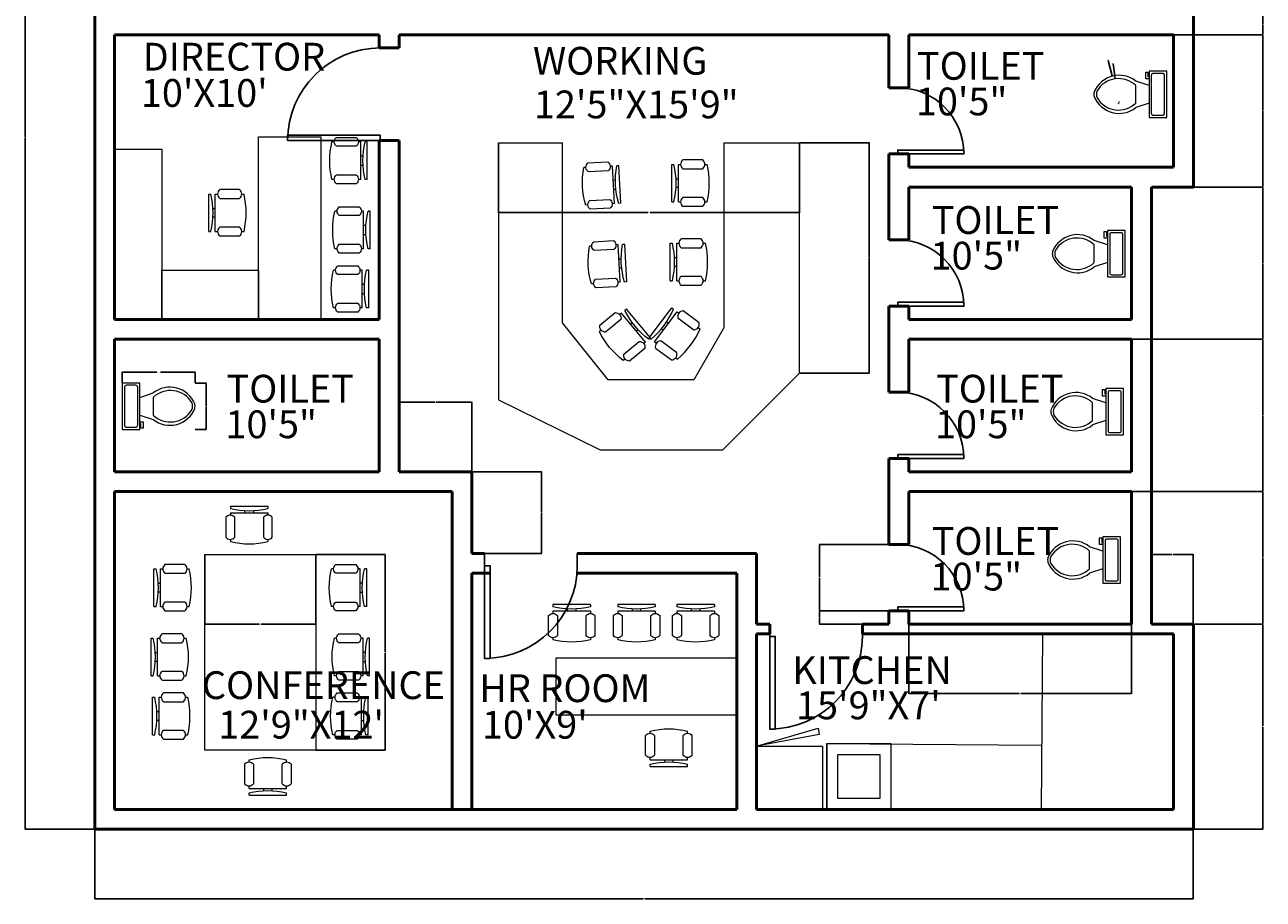
# Model space of a CAD drawing. Units: inches. Extents: x 4242 to 4803, y 4687 to 5377.
# Tile 1 of 2: x 4242 to 4803, y 4687 to 5083. Entities that reach past the tile are written whole.
import ezdxf

# ---------------------------------------------------------------- set-up
doc = ezdxf.new("R2010")
doc.units = ezdxf.units.IN
for name, color, linetype, lineweight in [('A-ANNO-DIMS', 2, 'Continuous', 18), ('A-AREA-IDEN', 7, 'Continuous', 25), ('A-DOOR', 4, 'Continuous', 25), ('A-FLOR-FIXT', 9, 'Continuous', 18), ('A-FURN', 8, 'Continuous', 18), ('A-WALL', 7, 'Continuous', 50)]:
    doc.layers.add(name, color=color, linetype=linetype, lineweight=lineweight)
doc.styles.get("Standard").update_dxf_attribs({"font": 'arial.ttf'})
doc.dimstyles.get("Standard").update_dxf_attribs({"dimtxt": 0.18, "dimasz": 0.18, "dimexe": 0.18, "dimexo": 0.0625, "dimgap": 0.09, "dimtad": 0, "dimtih": 1, "dimtoh": 1, "dimdec": 4, "dimzin": 0, "dimdsep": 46, "dimtxsty": 'Standard', "dimcen": 0.09, "dimadec": 0, "dimazin": 0, "dimtfac": 1, "dimtdec": 4, "dimtofl": 0, "dimtmove": 0, "dimatfit": 3, "dimfxl": 1, "dimtolj": 1, "dimtzin": 0, "dimarcsym": 0})

# ---------------------------------------------------------------- blocks, each defined once
blk = doc.blocks.new('Toilet - top')
for p, q in [((9.5, -6), (9.5, -2)), ((-10, -8.5), (-8, -8.5)), ((-10, -9.5), (-10, -8.5)), ((-7, -9.5), (-10, -9.5)), ((-8, -8.5), (-8, -8)), ((-7, -8), (-7, -9.5)), ((-4, -8), (-6, -14)), ((4, -8), (6, -14)), ((4, -14), (-4, -14))]:
    blk.add_line(p, q)
blk.add_lwpolyline([(10.5, -8), (10.5, 0), (-10.5, 0), (-10.5, -8)], close=True)
for points in [[(-9.5, -2), (-9.5, -6)], [(8.5, -1), (-8.5, -1)], [(-8.5, -7), (8.5, -7)]]:
    blk.add_lwpolyline(points)
for centre, radius, start, end in [((-8.62, -1.88), 0.884, 81.8699, 188.1301), ((8.62, -1.88), 0.884, 351.8699, 98.1301), ((-8.62, -6.12), 0.884, 171.8699, 278.1301), ((8.62, -6.12), 0.884, 261.8699, 8.1301), ((3.52, -21.58), 12.17, 141.4691, 247.9714), ((4.2, -21.82), 11.33, 136.3677, 238.9468), ((-3.52, -21.58), 12.17, 292.0284, 38.5307), ((-4.2, -21.82), 11.33, 301.053, 43.6321), ((0, -27.88), 4, 245.7318, 294.2682), ((0, -29), 4, 254.8605, 285.1395)]:
    blk.add_arc(centre, radius, start, end)
blk = doc.blocks.new('Chair - Desk')
for p, q in [((-8.5, 0), (-8.5, -1)), ((-8.5, 0), (8.5, 0)), ((8.5, 0), (8.5, -1)), ((-10.5, -5), (-10.5, -14)), ((-8.5, -3), (-8.5, -4)), ((-8.5, -3), (8.5, -3)), ((-6.5, -14), (-6.5, -5)), ((-2, -3), (-2, -1.9355)), ((2, -1.9576), (2, -3)), ((6.5, -5), (6.5, -14)), ((8.5, -3), (8.5, -4)), ((10.5, -14), (10.5, -5)), ((-8.5, -15), (-8.5, -16)), ((8.5, -15), (8.5, -16))]:
    blk.add_line(p, q)
for centre, radius, start, end in [((-8.5, -6.5), 2.5, 36.8699, 143.1301), ((0, 34.625), 36.625, 256.5803, 283.4197), ((8.5, -6.5), 2.5, 36.8699, 143.1301), ((-8.5, -12.5), 2.5, 216.8699, 323.1301), ((0, 19.625), 36.625, 256.5803, 283.4197), ((8.5, -12.5), 2.5, 216.8699, 323.1301)]:
    blk.add_arc(centre, radius, start, end)
blk = doc.blocks.new('*U4')
for p, q in [((0, 0), (0, -100)), ((750, 0), (750, -100))]:
    blk.add_line(p, q)
blk.add_lwpolyline([(0, 0), (0, 750), (43.75, 750), (43.75, 0)], close=True)
blk.add_arc((0, 0), 750, 0, 90)
blk = doc.blocks.new('*D8')
at = {"layer": 'A-ANNO-DIMS', "color": 0, "lineweight": -2, "transparency": 16777216}
for p, q in [((4285.76, 4920.88), (4285.76, 4925.95)), ((4285.94, 4925.77), (4301.51, 4925.77)), ((4318.63, 4925.77), (4303.06, 4925.77)), ((4318.81, 4920.88), (4318.81, 4925.95))]:
    blk.add_line(p, q, dxfattribs=at)
at = {"layer": 'A-ANNO-DIMS', "color": 0, "transparency": 16777216}
for points in [[(4285.94, 4925.8), (4285.94, 4925.74), (4285.76, 4925.77)], [(4318.63, 4925.8), (4318.63, 4925.74), (4318.81, 4925.77)]]:
    blk.add_solid(points, dxfattribs=at)
at = {"layer": 'Defpoints', "color": 0, "transparency": 16777216}
for p in [(4285.76, 4925.77), (4285.76, 4920.82), (4318.81, 4920.82)]:
    blk.add_point(p, dxfattribs=at)
at = {"layer": 'A-ANNO-DIMS', "color": 0, "transparency": 16777216, "insert": (4302.29, 4925.77), "char_height": 0.18, "attachment_point": 5}
blk.add_mtext('\\A1;WC 33 TYP.', dxfattribs=at)
blk = doc.blocks.new('*D9')
at = {"layer": 'A-ANNO-DIMS', "color": 0, "lineweight": -2, "transparency": 16777216}
for p, q in [((4318.87, 4920.82), (4323.95, 4920.82)), ((4323.77, 4920.64), (4323.77, 4910.5)), ((4323.77, 4900), (4323.77, 4910.14)), ((4318.87, 4899.82), (4323.95, 4899.82))]:
    blk.add_line(p, q, dxfattribs=at)
at = {"layer": 'A-ANNO-DIMS', "color": 0, "transparency": 16777216}
for points in [[(4323.74, 4920.64), (4323.8, 4920.64), (4323.77, 4920.82)], [(4323.74, 4900), (4323.8, 4900), (4323.77, 4899.82)]]:
    blk.add_solid(points, dxfattribs=at)
at = {"layer": 'Defpoints', "color": 0, "transparency": 16777216}
for p in [(4318.81, 4920.82), (4323.77, 4920.82), (4318.81, 4899.82)]:
    blk.add_point(p, dxfattribs=at)
at = {"layer": 'A-ANNO-DIMS', "color": 0, "transparency": 16777216, "insert": (4323.77, 4910.32), "char_height": 0.18, "attachment_point": 5}
blk.add_mtext('\\A1;21 TYP.', dxfattribs=at)
blk = doc.blocks.new('*D12')
at = {"layer": 'A-ANNO-DIMS', "color": 0, "lineweight": -2, "transparency": 16777216}
for p, q in [((4273.28, 4718.58), (4273.28, 4686.96)), ((4771.28, 4718.58), (4771.28, 4686.96)), ((4273.46, 4687.14), (4521.99, 4687.14)), ((4771.1, 4687.14), (4522.58, 4687.14))]:
    blk.add_line(p, q, dxfattribs=at)
at = {"layer": 'A-ANNO-DIMS', "color": 0, "transparency": 16777216}
for points in [[(4273.46, 4687.17), (4273.46, 4687.11), (4273.28, 4687.14)], [(4771.1, 4687.17), (4771.1, 4687.11), (4771.28, 4687.14)]]:
    blk.add_solid(points, dxfattribs=at)
at = {"layer": 'Defpoints', "color": 0, "transparency": 16777216}
for p in [(4273.28, 4718.64), (4771.28, 4718.64), (4771.28, 4687.14)]:
    blk.add_point(p, dxfattribs=at)
at = {"layer": 'A-ANNO-DIMS', "color": 0, "transparency": 16777216, "insert": (4522.28, 4687.14), "char_height": 0.18, "attachment_point": 5}
blk.add_mtext('\\A1;498', dxfattribs=at)
blk = doc.blocks.new('*D13')
at = {"layer": 'A-ANNO-DIMS', "color": 0, "lineweight": -2, "transparency": 16777216}
for p, q in [((4633.22, 5345.64), (4241.6, 5345.64)), ((4241.78, 5345.46), (4241.78, 5032.32)), ((4241.78, 4718.82), (4241.78, 5031.96)), ((4273.22, 4718.64), (4241.6, 4718.64))]:
    blk.add_line(p, q, dxfattribs=at)
at = {"layer": 'A-ANNO-DIMS', "color": 0, "transparency": 16777216}
for points in [[(4241.75, 5345.46), (4241.81, 5345.46), (4241.78, 5345.64)], [(4241.75, 4718.82), (4241.81, 4718.82), (4241.78, 4718.64)]]:
    blk.add_solid(points, dxfattribs=at)
at = {"layer": 'Defpoints', "color": 0, "transparency": 16777216}
for p in [(4241.78, 5345.64), (4633.28, 5345.64), (4273.28, 4718.64)]:
    blk.add_point(p, dxfattribs=at)
at = {"layer": 'A-ANNO-DIMS', "color": 0, "transparency": 16777216, "insert": (4241.78, 5032.14), "char_height": 0.18, "attachment_point": 5}
blk.add_mtext('\\A1;627', dxfattribs=at)
blk = doc.blocks.new('*D16')
at = {"layer": 'A-ANNO-DIMS', "color": 0, "lineweight": -2, "transparency": 16777216}
for p, q in [((4771.35, 4811.64), (4802.96, 4811.64)), ((4802.78, 4811.46), (4802.78, 4765.32)), ((4802.78, 4718.82), (4802.78, 4764.96)), ((4771.35, 4718.64), (4802.96, 4718.64))]:
    blk.add_line(p, q, dxfattribs=at)
at = {"layer": 'A-ANNO-DIMS', "color": 0, "transparency": 16777216}
for points in [[(4802.75, 4811.46), (4802.81, 4811.46), (4802.78, 4811.64)], [(4802.75, 4718.82), (4802.81, 4718.82), (4802.78, 4718.64)]]:
    blk.add_solid(points, dxfattribs=at)
at = {"layer": 'Defpoints', "color": 0, "transparency": 16777216}
for p in [(4771.28, 4811.64), (4802.78, 4811.64), (4771.28, 4718.64)]:
    blk.add_point(p, dxfattribs=at)
at = {"layer": 'A-ANNO-DIMS', "color": 0, "transparency": 16777216, "insert": (4802.78, 4765.14), "char_height": 0.18, "attachment_point": 5}
blk.add_mtext('\\A1;93', dxfattribs=at)
blk = doc.blocks.new('*D17')
at = {"layer": 'A-ANNO-DIMS', "color": 0, "lineweight": -2, "transparency": 16777216}
for p, q in [((4743.35, 4871.64), (4802.96, 4871.64)), ((4802.78, 4871.46), (4802.78, 4841.82)), ((4802.78, 4811.82), (4802.78, 4841.46)), ((4752.35, 4811.64), (4802.96, 4811.64))]:
    blk.add_line(p, q, dxfattribs=at)
at = {"layer": 'A-ANNO-DIMS', "color": 0, "transparency": 16777216}
for points in [[(4802.75, 4871.46), (4802.81, 4871.46), (4802.78, 4871.64)], [(4802.75, 4811.82), (4802.81, 4811.82), (4802.78, 4811.64)]]:
    blk.add_solid(points, dxfattribs=at)
at = {"layer": 'Defpoints', "color": 0, "transparency": 16777216}
for p in [(4743.28, 4871.64), (4802.78, 4871.64), (4752.28, 4811.64)]:
    blk.add_point(p, dxfattribs=at)
at = {"layer": 'A-ANNO-DIMS', "color": 0, "transparency": 16777216, "insert": (4802.78, 4841.64), "char_height": 0.18, "attachment_point": 5}
blk.add_mtext('\\A1;60', dxfattribs=at)
blk = doc.blocks.new('*D18')
at = {"layer": 'A-ANNO-DIMS', "color": 0, "lineweight": -2, "transparency": 16777216}
for p, q in [((4743.35, 4940.64), (4802.96, 4940.64)), ((4802.78, 4940.46), (4802.78, 4906.32)), ((4802.78, 4871.82), (4802.78, 4905.96)), ((4743.35, 4871.64), (4802.96, 4871.64))]:
    blk.add_line(p, q, dxfattribs=at)
at = {"layer": 'A-ANNO-DIMS', "color": 0, "transparency": 16777216}
for points in [[(4802.75, 4940.46), (4802.81, 4940.46), (4802.78, 4940.64)], [(4802.75, 4871.82), (4802.81, 4871.82), (4802.78, 4871.64)]]:
    blk.add_solid(points, dxfattribs=at)
at = {"layer": 'Defpoints', "color": 0, "transparency": 16777216}
for p in [(4743.28, 4940.64), (4802.78, 4940.64), (4743.28, 4871.64)]:
    blk.add_point(p, dxfattribs=at)
at = {"layer": 'A-ANNO-DIMS', "color": 0, "transparency": 16777216, "insert": (4802.78, 4906.14), "char_height": 0.18, "attachment_point": 5}
blk.add_mtext('\\A1;69', dxfattribs=at)
blk = doc.blocks.new('*D19')
at = {"layer": 'A-ANNO-DIMS', "color": 0, "lineweight": -2, "transparency": 16777216}
for p, q in [((4752.35, 5009.64), (4802.96, 5009.64)), ((4802.78, 5009.46), (4802.78, 4975.32)), ((4802.78, 4940.82), (4802.78, 4974.96)), ((4743.35, 4940.64), (4802.96, 4940.64))]:
    blk.add_line(p, q, dxfattribs=at)
at = {"layer": 'A-ANNO-DIMS', "color": 0, "transparency": 16777216}
for points in [[(4802.75, 5009.46), (4802.81, 5009.46), (4802.78, 5009.64)], [(4802.75, 4940.82), (4802.81, 4940.82), (4802.78, 4940.64)]]:
    blk.add_solid(points, dxfattribs=at)
at = {"layer": 'Defpoints', "color": 0, "transparency": 16777216}
for p in [(4752.28, 5009.64), (4802.78, 5009.64), (4743.28, 4940.64)]:
    blk.add_point(p, dxfattribs=at)
at = {"layer": 'A-ANNO-DIMS', "color": 0, "transparency": 16777216, "insert": (4802.78, 4975.14), "char_height": 0.18, "attachment_point": 5}
blk.add_mtext('\\A1;69', dxfattribs=at)
blk = doc.blocks.new('*D20')
at = {"layer": 'A-ANNO-DIMS', "color": 0, "lineweight": -2, "transparency": 16777216}
for p, q in [((4762.35, 5078.64), (4802.96, 5078.64)), ((4802.78, 5078.46), (4802.78, 5044.32)), ((4802.78, 5009.82), (4802.78, 5043.96)), ((4771.35, 5009.64), (4802.96, 5009.64))]:
    blk.add_line(p, q, dxfattribs=at)
at = {"layer": 'A-ANNO-DIMS', "color": 0, "transparency": 16777216}
for points in [[(4802.75, 5078.46), (4802.81, 5078.46), (4802.78, 5078.64)], [(4802.75, 5009.82), (4802.81, 5009.82), (4802.78, 5009.64)]]:
    blk.add_solid(points, dxfattribs=at)
at = {"layer": 'Defpoints', "color": 0, "transparency": 16777216}
for p in [(4762.28, 5078.64), (4802.78, 5078.64), (4771.28, 5009.64)]:
    blk.add_point(p, dxfattribs=at)
at = {"layer": 'A-ANNO-DIMS', "color": 0, "transparency": 16777216, "insert": (4802.78, 5044.14), "char_height": 0.18, "attachment_point": 5}
blk.add_mtext('\\A1;69', dxfattribs=at)
blk = doc.blocks.new('*D21')
at = {"layer": 'A-ANNO-DIMS', "color": 0, "lineweight": -2, "transparency": 16777216}
for p, q in [((4762.35, 5087.64), (4802.96, 5087.64)), ((4802.78, 5087.46), (4802.78, 5083.32)), ((4802.78, 5078.82), (4802.78, 5082.96)), ((4762.35, 5078.64), (4802.96, 5078.64))]:
    blk.add_line(p, q, dxfattribs=at)
at = {"layer": 'A-ANNO-DIMS', "color": 0, "transparency": 16777216}
for points in [[(4802.75, 5087.46), (4802.81, 5087.46), (4802.78, 5087.64)], [(4802.75, 5078.82), (4802.81, 5078.82), (4802.78, 5078.64)]]:
    blk.add_solid(points, dxfattribs=at)
at = {"layer": 'Defpoints', "color": 0, "transparency": 16777216}
for p in [(4762.28, 5087.64), (4802.78, 5087.64), (4762.28, 5078.64)]:
    blk.add_point(p, dxfattribs=at)
at = {"layer": 'A-ANNO-DIMS', "color": 0, "transparency": 16777216, "insert": (4802.78, 5083.14), "char_height": 0.18, "attachment_point": 5}
blk.add_mtext('\\A1;9', dxfattribs=at)
blk = doc.blocks.new('*D25')
at = {"layer": 'A-ANNO-DIMS', "color": 0, "lineweight": -2, "transparency": 16777216}
for p, q in [((4752.28, 4811.7), (4752.28, 4843.32)), ((4752.46, 4843.14), (4761.57, 4843.14)), ((4771.1, 4843.14), (4762, 4843.14)), ((4771.28, 4811.7), (4771.28, 4843.32))]:
    blk.add_line(p, q, dxfattribs=at)
at = {"layer": 'A-ANNO-DIMS', "color": 0, "transparency": 16777216}
for points in [[(4752.46, 4843.17), (4752.46, 4843.11), (4752.28, 4843.14)], [(4771.1, 4843.17), (4771.1, 4843.11), (4771.28, 4843.14)]]:
    blk.add_solid(points, dxfattribs=at)
at = {"layer": 'Defpoints', "color": 0, "transparency": 16777216}
for p in [(4771.28, 4843.14), (4752.28, 4811.64), (4771.28, 4811.64)]:
    blk.add_point(p, dxfattribs=at)
at = {"layer": 'A-ANNO-DIMS', "color": 0, "transparency": 16777216, "insert": (4761.78, 4843.14), "char_height": 0.18, "attachment_point": 5}
blk.add_mtext('\\A1;19', dxfattribs=at)
blk = doc.blocks.new('*D28')
at = {"layer": 'A-ANNO-DIMS', "color": 0, "lineweight": -2, "transparency": 16777216}
for p, q in [((4633.22, 4847.64), (4601.6, 4847.64)), ((4601.78, 4847.46), (4601.78, 4832.82)), ((4601.78, 4817.82), (4601.78, 4832.46)), ((4633.22, 4817.64), (4601.6, 4817.64))]:
    blk.add_line(p, q, dxfattribs=at)
at = {"layer": 'A-ANNO-DIMS', "color": 0, "transparency": 16777216}
for points in [[(4601.75, 4847.46), (4601.81, 4847.46), (4601.78, 4847.64)], [(4601.75, 4817.82), (4601.81, 4817.82), (4601.78, 4817.64)]]:
    blk.add_solid(points, dxfattribs=at)
at = {"layer": 'Defpoints', "color": 0, "transparency": 16777216}
for p in [(4601.78, 4847.64), (4633.28, 4847.64), (4633.28, 4817.64)]:
    blk.add_point(p, dxfattribs=at)
at = {"layer": 'A-ANNO-DIMS', "color": 0, "transparency": 16777216, "insert": (4601.78, 4832.64), "char_height": 0.18, "attachment_point": 5}
blk.add_mtext('\\A1;30', dxfattribs=at)
blk = doc.blocks.new('*D29')
at = {"layer": 'A-ANNO-DIMS', "color": 0, "lineweight": -2, "transparency": 16777216}
for p, q in [((4633.22, 4817.64), (4601.6, 4817.64)), ((4601.78, 4817.46), (4601.78, 4814.82)), ((4633.22, 4811.64), (4601.6, 4811.64)), ((4601.78, 4811.82), (4601.78, 4814.46))]:
    blk.add_line(p, q, dxfattribs=at)
at = {"layer": 'A-ANNO-DIMS', "color": 0, "transparency": 16777216}
for points in [[(4601.75, 4817.46), (4601.81, 4817.46), (4601.78, 4817.64)], [(4601.75, 4811.82), (4601.81, 4811.82), (4601.78, 4811.64)]]:
    blk.add_solid(points, dxfattribs=at)
at = {"layer": 'Defpoints', "color": 0, "transparency": 16777216}
for p in [(4601.78, 4817.64), (4633.28, 4817.64), (4633.28, 4811.64)]:
    blk.add_point(p, dxfattribs=at)
at = {"layer": 'A-ANNO-DIMS', "color": 0, "transparency": 16777216, "insert": (4601.78, 4814.64), "char_height": 0.18, "attachment_point": 5}
blk.add_mtext('\\A1;6', dxfattribs=at)
blk = doc.blocks.new('*D32')
at = {"layer": 'A-ANNO-DIMS', "color": 0, "lineweight": -2, "transparency": 16777216}
for p, q in [((4642.28, 4811.58), (4642.28, 4779.96)), ((4743.28, 4811.58), (4743.28, 4779.96)), ((4642.46, 4780.14), (4692.52, 4780.14)), ((4743.1, 4780.14), (4693.05, 4780.14))]:
    blk.add_line(p, q, dxfattribs=at)
at = {"layer": 'A-ANNO-DIMS', "color": 0, "transparency": 16777216}
for points in [[(4642.46, 4780.17), (4642.46, 4780.11), (4642.28, 4780.14)], [(4743.1, 4780.17), (4743.1, 4780.11), (4743.28, 4780.14)]]:
    blk.add_solid(points, dxfattribs=at)
at = {"layer": 'Defpoints', "color": 0, "transparency": 16777216}
for p in [(4642.28, 4811.64), (4743.28, 4811.64), (4642.28, 4780.14)]:
    blk.add_point(p, dxfattribs=at)
at = {"layer": 'A-ANNO-DIMS', "color": 0, "transparency": 16777216, "insert": (4692.78, 4780.14), "char_height": 0.18, "attachment_point": 5}
blk.add_mtext('\\A1;101', dxfattribs=at)
blk = doc.blocks.new('*D33')
at = {"layer": 'A-ANNO-DIMS', "color": 0, "lineweight": -2, "transparency": 16777216}
for p, q in [((4411.28, 4880.7), (4411.28, 4912.32)), ((4411.46, 4912.14), (4427.57, 4912.14)), ((4444.1, 4912.14), (4428, 4912.14)), ((4444.28, 4880.7), (4444.28, 4912.32))]:
    blk.add_line(p, q, dxfattribs=at)
at = {"layer": 'A-ANNO-DIMS', "color": 0, "transparency": 16777216}
for points in [[(4411.46, 4912.17), (4411.46, 4912.11), (4411.28, 4912.14)], [(4444.1, 4912.17), (4444.1, 4912.11), (4444.28, 4912.14)]]:
    blk.add_solid(points, dxfattribs=at)
at = {"layer": 'Defpoints', "color": 0, "transparency": 16777216}
for p in [(4444.28, 4912.14), (4411.28, 4880.64), (4444.28, 4880.64)]:
    blk.add_point(p, dxfattribs=at)
at = {"layer": 'A-ANNO-DIMS', "color": 0, "transparency": 16777216, "insert": (4427.78, 4912.14), "char_height": 0.18, "attachment_point": 5}
blk.add_mtext('\\A1;33', dxfattribs=at)
blk = doc.blocks.new('*D34')
at = {"layer": 'A-ANNO-DIMS', "color": 0, "lineweight": -2, "transparency": 16777216}
for p, q in [((4444.35, 4880.64), (4475.96, 4880.64)), ((4475.78, 4880.46), (4475.78, 4862.32)), ((4475.78, 4843.82), (4475.78, 4861.96)), ((4444.35, 4843.64), (4475.96, 4843.64))]:
    blk.add_line(p, q, dxfattribs=at)
at = {"layer": 'A-ANNO-DIMS', "color": 0, "transparency": 16777216}
for points in [[(4475.75, 4880.46), (4475.81, 4880.46), (4475.78, 4880.64)], [(4475.75, 4843.82), (4475.81, 4843.82), (4475.78, 4843.64)]]:
    blk.add_solid(points, dxfattribs=at)
at = {"layer": 'Defpoints', "color": 0, "transparency": 16777216}
for p in [(4444.28, 4880.64), (4444.28, 4843.64), (4475.78, 4843.64)]:
    blk.add_point(p, dxfattribs=at)
at = {"layer": 'A-ANNO-DIMS', "color": 0, "transparency": 16777216, "insert": (4475.78, 4862.14), "char_height": 0.18, "attachment_point": 5}
blk.add_mtext('\\A1;37', dxfattribs=at)
blk = doc.blocks.new('*D35')
at = {"layer": 'A-ANNO-DIMS', "color": 0, "lineweight": -2, "transparency": 16777216}
for p, q in [((4456.34, 5029.6), (4456.34, 4997.98)), ((4592.78, 5029.6), (4592.78, 4997.98)), ((4456.52, 4998.16), (4524.1, 4998.16)), ((4592.6, 4998.16), (4525.01, 4998.16))]:
    blk.add_line(p, q, dxfattribs=at)
at = {"layer": 'A-ANNO-DIMS', "color": 0, "transparency": 16777216}
for points in [[(4456.52, 4998.19), (4456.52, 4998.13), (4456.34, 4998.16)], [(4592.6, 4998.19), (4592.6, 4998.13), (4592.78, 4998.16)]]:
    blk.add_solid(points, dxfattribs=at)
at = {"layer": 'Defpoints', "color": 0, "transparency": 16777216}
for p in [(4456.34, 5029.66), (4592.78, 5029.66), (4456.34, 4998.16)]:
    blk.add_point(p, dxfattribs=at)
at = {"layer": 'A-ANNO-DIMS', "color": 0, "transparency": 16777216, "insert": (4524.56, 4998.16), "char_height": 0.18, "attachment_point": 5}
blk.add_mtext('\\A1;136.44', dxfattribs=at)
blk = doc.blocks.new('*D36')
at = {"layer": 'A-ANNO-DIMS', "color": 0, "lineweight": -2, "transparency": 16777216}
for p, q in [((4592.84, 5029.66), (4624.46, 5029.66)), ((4624.28, 5029.48), (4624.28, 4977.7)), ((4624.28, 4925.55), (4624.28, 4977.33)), ((4592.84, 4925.37), (4624.46, 4925.37))]:
    blk.add_line(p, q, dxfattribs=at)
at = {"layer": 'A-ANNO-DIMS', "color": 0, "transparency": 16777216}
for points in [[(4624.25, 5029.48), (4624.31, 5029.48), (4624.28, 5029.66)], [(4624.25, 4925.55), (4624.31, 4925.55), (4624.28, 4925.37)]]:
    blk.add_solid(points, dxfattribs=at)
at = {"layer": 'Defpoints', "color": 0, "transparency": 16777216}
for p in [(4592.78, 5029.66), (4592.78, 4925.37), (4624.28, 4925.37)]:
    blk.add_point(p, dxfattribs=at)
at = {"layer": 'A-ANNO-DIMS', "color": 0, "transparency": 16777216, "insert": (4624.28, 4977.52), "char_height": 0.18, "attachment_point": 5}
blk.add_mtext('\\A1;104.29', dxfattribs=at)
blk = doc.blocks.new('*D39')
at = {"layer": 'A-ANNO-DIMS', "color": 0, "lineweight": -2, "transparency": 16777216}
for p, q in [((4323.22, 4843.02), (4323.22, 4811.4)), ((4373.49, 4843.02), (4373.49, 4811.4)), ((4323.4, 4811.58), (4347.96, 4811.58)), ((4373.31, 4811.58), (4348.75, 4811.58))]:
    blk.add_line(p, q, dxfattribs=at)
at = {"layer": 'A-ANNO-DIMS', "color": 0, "transparency": 16777216}
for points in [[(4323.4, 4811.61), (4323.4, 4811.55), (4323.22, 4811.58)], [(4373.31, 4811.61), (4373.31, 4811.55), (4373.49, 4811.58)]]:
    blk.add_solid(points, dxfattribs=at)
at = {"layer": 'Defpoints', "color": 0, "transparency": 16777216}
for p in [(4323.22, 4843.08), (4373.49, 4843.08), (4323.22, 4811.58)]:
    blk.add_point(p, dxfattribs=at)
at = {"layer": 'A-ANNO-DIMS', "color": 0, "transparency": 16777216, "insert": (4348.36, 4811.58), "char_height": 0.18, "attachment_point": 5}
blk.add_mtext('\\A1;50.28', dxfattribs=at)
blk = doc.blocks.new('*D40')
at = {"layer": 'A-ANNO-DIMS', "color": 0, "lineweight": -2, "transparency": 16777216}
for p, q in [((4373.56, 4843.08), (4405.17, 4843.08)), ((4404.99, 4842.9), (4404.99, 4798.98)), ((4404.99, 4754.7), (4404.99, 4798.62)), ((4373.56, 4754.52), (4405.17, 4754.52))]:
    blk.add_line(p, q, dxfattribs=at)
at = {"layer": 'A-ANNO-DIMS', "color": 0, "transparency": 16777216}
for points in [[(4404.96, 4842.9), (4405.02, 4842.9), (4404.99, 4843.08)], [(4404.96, 4754.7), (4405.02, 4754.7), (4404.99, 4754.52)]]:
    blk.add_solid(points, dxfattribs=at)
at = {"layer": 'Defpoints', "color": 0, "transparency": 16777216}
for p in [(4373.49, 4843.08), (4373.49, 4754.52), (4404.99, 4754.52)]:
    blk.add_point(p, dxfattribs=at)
at = {"layer": 'A-ANNO-DIMS', "color": 0, "transparency": 16777216, "insert": (4404.99, 4798.8), "char_height": 0.18, "attachment_point": 5}
blk.add_mtext('\\A1;88.56', dxfattribs=at)
blk = doc.blocks.new('*D42')
at = {"layer": 'A-ANNO-DIMS', "color": 0, "lineweight": -2, "transparency": 16777216}
for p, q in [((4732.5, 5066.95), (4732.68, 5066.95)), ((4732.68, 5066.95), (4734.49, 5060.06)), ((4737.54, 5048.12), (4737.72, 5048.12)), ((4737.63, 5048.03), (4737.63, 5048.21))]:
    blk.add_line(p, q, dxfattribs=at)
at = {"layer": 'A-ANNO-DIMS', "color": 0, "transparency": 16777216}
blk.add_solid([(4734.52, 5060.07), (4734.46, 5060.06), (4734.53, 5059.89)], dxfattribs=at)
at = {"layer": 'Defpoints', "color": 0, "transparency": 16777216}
for p in [(4734.53, 5059.89), (4737.63, 5048.12)]:
    blk.add_point(p, dxfattribs=at)
at = {"layer": 'A-ANNO-DIMS', "color": 0, "transparency": 16777216, "insert": (4731.76, 5066.95), "char_height": 0.18, "attachment_point": 5}
blk.add_mtext('\\A1;10X R12.17', dxfattribs=at)
blk = doc.blocks.new('*D43')
at = {"layer": 'A-ANNO-DIMS', "color": 0, "lineweight": -2, "transparency": 16777216}
for p, q in [((4734.79, 5065.4), (4734.97, 5065.4)), ((4734.97, 5065.4), (4735.86, 5058.85)), ((4737.3, 5047.44), (4737.48, 5047.44)), ((4737.39, 5047.35), (4737.39, 5047.53))]:
    blk.add_line(p, q, dxfattribs=at)
at = {"layer": 'A-ANNO-DIMS', "color": 0, "transparency": 16777216}
blk.add_solid([(4735.88, 5058.85), (4735.83, 5058.84), (4735.88, 5058.67)], dxfattribs=at)
at = {"layer": 'Defpoints', "color": 0, "transparency": 16777216}
for p in [(4735.88, 5058.67), (4737.39, 5047.44)]:
    blk.add_point(p, dxfattribs=at)
at = {"layer": 'A-ANNO-DIMS', "color": 0, "transparency": 16777216, "insert": (4734.06, 5065.4), "char_height": 0.18, "attachment_point": 5}
blk.add_mtext('\\A1;10X R11.33', dxfattribs=at)

msp = doc.modelspace()

# ---------------------------------------------------------------- linework, layer by layer
at = {"layer": 'A-FLOR-FIXT'}
for p, q in [((4702.9438, 4807.1424), (4702.2844, 4727.6424)), ((4573.2844, 4756.2338), (4601.25, 4764.4402)), ((4601.6435, 4761.6002), (4573.2844, 4756.2338)), ((4601.25, 4764.4402), (4601.6435, 4761.6002)), ((4605.1756, 4757.5105), (4702.5255, 4756.7031)), ((4605.1756, 4757.5105), (4605.1756, 4727.6424))]:
    msp.add_line(p, q, dxfattribs=at)
for points in [[(4573.2844, 4756.2338), (4603.1574, 4756.2338), (4603.1574, 4727.6424), (4573.2844, 4727.6424)], [(4605.1756, 4757.5105), (4634.108, 4757.5105), (4634.108, 4727.6424), (4605.1756, 4727.6424)], [(4610.1756, 4752.5105), (4629.108, 4752.5105), (4629.108, 4732.6424), (4610.1756, 4732.6424)]]:
    msp.add_lwpolyline(points, close=True, dxfattribs=at)
at = {"layer": 'A-FURN'}
for p, q in [((4456.3394, 5029.6591), (4456.3394, 4913.1566)), ((4456.3394, 5029.6591), (4485.3365, 5029.6591)), ((4485.3365, 4948.1746), (4485.3365, 5029.6591)), ((4558.4804, 5029.6591), (4558.4804, 4945.818)), ((4558.4804, 5029.6591), (4592.7788, 5029.6591)), ((4592.7788, 4925.374), (4592.7788, 5029.6591)), ((4505.982, 4922.2522), (4485.3365, 4948.1746)), ((4558.4804, 4945.818), (4544.9133, 4922.2522)), ((4557.9632, 4890.6012), (4592.7788, 4925.374)), ((4544.9133, 4922.2522), (4505.982, 4922.2522)), ((4456.3394, 4913.1566), (4502.4465, 4890.6012)), ((4502.4465, 4890.6012), (4557.9632, 4890.6012))]:
    msp.add_line(p, q, dxfattribs=at)
for points in [[(4347.5675, 5032.3028), (4375.8189, 5032.3028), (4375.8189, 4949.6424), (4347.5675, 4949.6424)], [(4282.2844, 5026.853), (4303.6738, 5026.853), (4303.6738, 4949.6424), (4282.2844, 4949.6424)], [(4303.6738, 4971.9217), (4347.5675, 4971.9217), (4347.5675, 4949.6424), (4303.6738, 4949.6424)], [(4323.2168, 4843.0795), (4373.4937, 4843.0795), (4373.4937, 4754.5187), (4323.2168, 4754.5187)], [(4482.445, 4796.2999), (4564.2844, 4796.2999), (4564.2844, 4770.3297), (4482.445, 4770.3297)]]:
    msp.add_lwpolyline(points, close=True, dxfattribs=at)
at = {"layer": 'A-WALL'}
for p, q in [((4771.2844, 5345.6424), (4771.2844, 5009.6424)), ((4273.2844, 5231.6424), (4273.2844, 4718.6424)), ((4282.2844, 5078.6424), (4402.2844, 5078.6424)), ((4282.2844, 5078.6424), (4282.2844, 4949.6424)), ((4402.2844, 5078.6424), (4402.2844, 5072.6424)), ((4411.2844, 5078.6424), (4633.2844, 5078.6424)), ((4411.2844, 5078.6424), (4411.2844, 5072.6424)), ((4633.2844, 5078.6424), (4633.2844, 5054.6424)), ((4642.2844, 5078.6424), (4642.2844, 5054.6424)), ((4642.2844, 5078.6424), (4762.2844, 5078.6424)), ((4762.2844, 5078.6424), (4762.2844, 5018.6424)), ((4402.2844, 5072.6424), (4411.2844, 5072.6424)), ((4642.2844, 5054.6424), (4633.2844, 5054.6424)), ((4402.2844, 5030.6424), (4411.2844, 5030.6424)), ((4402.2844, 5030.6424), (4402.2844, 4949.6424)), ((4411.2844, 5030.6424), (4411.2844, 4880.6424)), ((4642.2844, 5024.6424), (4633.2844, 5024.6424)), ((4633.2844, 5024.6424), (4633.2844, 4985.6424)), ((4642.2844, 5024.6424), (4642.2844, 5018.6424)), ((4642.2844, 5018.6424), (4762.2844, 5018.6424)), ((4642.2844, 5009.6424), (4743.2844, 5009.6424)), ((4642.2844, 5009.6424), (4642.2844, 4985.6424)), ((4743.2844, 5009.6424), (4743.2844, 4949.6424)), ((4752.2844, 5009.6424), (4752.2844, 4811.6424)), ((4752.2844, 5009.6424), (4771.2844, 5009.6424)), ((4642.2844, 4985.6424), (4633.2844, 4985.6424)), ((4642.2844, 4955.6424), (4633.2844, 4955.6424)), ((4633.2844, 4955.6424), (4633.2844, 4916.6424)), ((4642.2844, 4955.6424), (4642.2844, 4949.6424)), ((4282.2844, 4949.6424), (4402.2844, 4949.6424)), ((4642.2844, 4949.6424), (4743.2844, 4949.6424)), ((4282.2844, 4940.6424), (4402.2844, 4940.6424)), ((4282.2844, 4940.6424), (4282.2844, 4880.6424)), ((4402.2844, 4940.6424), (4402.2844, 4880.6424)), ((4642.2844, 4940.6424), (4743.2844, 4940.6424)), ((4642.2844, 4940.6424), (4642.2844, 4916.6424)), ((4743.2844, 4940.6424), (4743.2844, 4880.6424)), ((4642.2844, 4916.6424), (4633.2844, 4916.6424)), ((4642.2844, 4886.6424), (4633.2844, 4886.6424)), ((4633.2844, 4886.6424), (4633.2844, 4847.6424)), ((4642.2844, 4886.6424), (4642.2844, 4880.6424)), ((4282.2844, 4880.6424), (4402.2844, 4880.6424)), ((4411.2844, 4880.6424), (4444.2844, 4880.6424)), ((4444.2844, 4880.6424), (4444.2844, 4843.6424)), ((4642.2844, 4880.6424), (4743.2844, 4880.6424)), ((4282.2844, 4871.6424), (4435.2844, 4871.6424)), ((4282.2844, 4871.6424), (4282.2844, 4727.6424)), ((4435.2844, 4871.6424), (4435.2844, 4727.6424)), ((4642.2844, 4871.6424), (4743.2844, 4871.6424)), ((4642.2844, 4871.6424), (4642.2844, 4847.6424)), ((4743.2844, 4871.6424), (4743.2844, 4811.6424)), ((4642.2844, 4847.6424), (4633.2844, 4847.6424)), ((4444.2844, 4843.6424), (4450.0155, 4843.6424)), ((4492.0155, 4843.6424), (4573.2844, 4843.6424)), ((4573.2844, 4843.6424), (4573.2844, 4811.6424)), ((4444.2844, 4834.6424), (4452.4655, 4834.6424)), ((4444.2844, 4834.6424), (4444.2844, 4727.6424)), ((4491.8777, 4834.6424), (4564.2844, 4834.6424)), ((4564.2844, 4834.6424), (4564.2844, 4727.6424)), ((4642.2844, 4817.6424), (4633.2844, 4817.6424)), ((4633.2844, 4817.6424), (4633.2844, 4811.6424)), ((4642.2844, 4817.6424), (4642.2844, 4811.6424)), ((4573.2844, 4811.6424), (4579.2844, 4811.6424)), ((4579.2844, 4811.6424), (4579.2844, 4807.1424)), ((4621.2844, 4811.6424), (4621.2844, 4807.1424)), ((4621.2844, 4811.6424), (4633.2844, 4811.6424)), ((4642.2844, 4811.6424), (4743.2844, 4811.6424)), ((4752.2844, 4811.6424), (4771.2844, 4811.6424)), ((4771.2844, 4811.6424), (4771.2844, 4718.6424)), ((4573.2844, 4807.1424), (4579.2844, 4807.1424)), ((4573.2844, 4807.1424), (4573.2844, 4727.6424)), ((4621.2844, 4807.1424), (4762.2844, 4807.1424)), ((4762.2844, 4807.1424), (4762.2844, 4727.6424)), ((4282.2844, 4727.6424), (4564.2844, 4727.6424)), ((4573.2844, 4727.6424), (4762.2844, 4727.6424)), ((4642.2844, 4727.6424), (4762.2844, 4727.6424)), ((4273.2844, 4718.6424), (4771.2844, 4718.6424))]:
    msp.add_line(p, q, dxfattribs=at)

# ---------------------------------------------------------------- block references
at = {"layer": 'A-DOOR'}
for p, xscale, yscale, zscale, rotation in [((4402.6885, 5030.6424), 0.0559999999999998, 0.0559999999999998, 0.0559999999999998, 90.00000000000003), ((4637.2844, 5024.6424), -0.0399999999999999, 0.0399999999999999, 0.0399999999999999, 270), ((4637.2844, 4955.6424), -0.0399999999999999, 0.0399999999999999, 0.0399999999999999, 270), ((4637.2844, 4886.6424), -0.0399999999999999, 0.0399999999999999, 0.0399999999999999, 270), ((4637.2844, 4817.6424), -0.0399999999999999, 0.0399999999999999, 0.0399999999999999, 270), ((4450.0155, 4838.0424), -0.0559999999999998, 0.0559999999999998, 0.0559999999999998, 180), ((4579.2844, 4806.0424), -0.0559999999999998, 0.0559999999999998, 0.0559999999999998, 180)]:
    msp.add_blockref('*U4', p, dxfattribs=dict(at, xscale=xscale, yscale=yscale, zscale=zscale, rotation=rotation))
at = {"layer": 'A-FLOR-FIXT'}
for p, rotation in [((4759.2061, 5051.6396), 270), ((4740.3562, 4979.4102), 270), ((4285.7638, 4910.3161), 89.99999999999999), ((4739.6418, 4907.8713), 270), ((4738.2505, 4840.6558), 270)]:
    msp.add_blockref('Toilet - top', p, dxfattribs=dict(at, rotation=rotation))
at = {"layer": 'A-FURN', "xscale": -1}
for p, rotation in [((4396.8396, 5021.6002), 270), ((4511.3759, 5010.7801), 272.9987426316156), ((4398.1678, 4990.1829), 270), ((4513.9909, 4975.1187), 272.9987426316156), ((4397.5042, 4963.4511), 270), ((4519.7974, 4947.8251), 309.6546020973546), ((4396.5755, 4828.1146), 270), ((4397.9037, 4796.6974), 270), ((4397.2401, 4769.9656), 270), ((4533.5126, 4747.1673), 180), ((4351.7836, 4734.1775), 180)]:
    msp.add_blockref('Chair - Desk', p, dxfattribs=dict(at, rotation=rotation))
at = {"layer": 'A-FURN'}
for p, rotation in [((4534.8689, 5011.395), 90), ((4324.9609, 4997.9519), 90), ((4534.123, 4975.6457), 90), ((4529.7523, 4948.0857), 53.34414053426098), ((4300.135, 4828.1146), 90), ((4298.8068, 4796.6974), 90), ((4299.4704, 4769.9656), 90)]:
    msp.add_blockref('Chair - Desk', p, dxfattribs=dict(at, rotation=rotation))
msp.add_blockref('Chair - Desk', (4343.2775, 4864.9866), dxfattribs=at)
at = {"layer": 'A-FURN', "xscale": -1}
for p in [(4489.5087, 4820.4479), (4518.8878, 4820.4479), (4545.6963, 4820.4479)]:
    msp.add_blockref('Chair - Desk', p, dxfattribs=at)

# ---------------------------------------------------------------- texts
at = {"layer": 'A-AREA-IDEN'}
for s, p in [('DIRECTOR', (4295.0324, 5062.3919)), ('WORKING', (4471.9338, 5060.5252)), ('TOILET', (4646.0082, 5058.2466)), ("10'X10'", (4294.2101, 5045.9654)), ('12\'5"X15\'9"', (4472.3462, 5040.759)), ('10\'5"', (4645.5032, 5042.1076)), ('TOILET', (4652.6702, 4988.3793)), ('10\'5"', (4652.1652, 4972.2404)), ('TOILET', (4333.046, 4911.9786)), ('TOILET', (4654.6654, 4911.9786)), ('10\'5"', (4332.541, 4895.8397)), ('10\'5"', (4654.1604, 4895.8397)), ('TOILET', (4652.6702, 4842.9786)), ('10\'5"', (4652.1652, 4826.8397)), ('KITCHEN', (4589.4857, 4784.4766)), ('CONFERENCE', (4321.8756, 4777.6483)), ('HR ROOM', (4447.5966, 4776.2651)), ('15\'9"X7\'', (4591.1831, 4768.4905)), ('12\'9"X12\'', (4329.2522, 4759.7512)), ("10'X9'", (4448.8096, 4759.7159))]:
    msp.add_text(s, height=12.5832, dxfattribs=at).set_placement(p)

# ---------------------------------------------------------------- dimensions: what is measured, and where the dimension line sits
at = {"layer": 'A-ANNO-DIMS'}
for base, p1, p2, angle, override, picture, middle in [((4241.7844, 5345.6424), (4273.2844, 4718.6424), (4633.2844, 5345.6424), 90, {"dimdec": 0, "dimlfac": 1, "dimrnd": 0, "dimzin": 0, "dimdsep": 46, "dimlunit": 2}, '*D13', (4241.7844, 5032.1424)), ((4802.7844, 5087.6424), (4762.2844, 5078.6424), (4762.2844, 5087.6424), 90, {"dimdec": 0, "dimlfac": 1, "dimrnd": 0, "dimzin": 0, "dimdsep": 46, "dimlunit": 2}, '*D21', (4802.7844, 5083.1424)), ((4802.7844, 5078.6424), (4771.2844, 5009.6424), (4762.2844, 5078.6424), 90, {"dimdec": 0, "dimlfac": 1, "dimrnd": 0, "dimzin": 0, "dimdsep": 46, "dimlunit": 2}, '*D20', (4802.7844, 5044.1424)), ((4456.3394, 4998.1591), (4592.7788, 5029.6591), (4456.3394, 5029.6591), 180, {"dimdec": 2, "dimlfac": 1, "dimrnd": 0, "dimzin": 0, "dimdsep": 46, "dimlunit": 2}, '*D35', (4524.5591, 4998.1591)), ((4624.2788, 4925.374), (4592.7788, 5029.6591), (4592.7788, 4925.374), 270, {"dimdec": 2, "dimlfac": 1, "dimrnd": 0, "dimzin": 0, "dimdsep": 46, "dimlunit": 2}, '*D36', (4624.2788, 4977.5165)), ((4802.7844, 5009.6424), (4743.2844, 4940.6424), (4752.2844, 5009.6424), 90, {"dimdec": 0, "dimlfac": 1, "dimrnd": 0, "dimzin": 0, "dimdsep": 46, "dimlunit": 2}, '*D19', (4802.7844, 4975.1424)), ((4802.7844, 4940.6424), (4743.2844, 4871.6424), (4743.2844, 4940.6424), 90, {"dimdec": 0, "dimlfac": 1, "dimrnd": 0, "dimzin": 0, "dimdsep": 46, "dimlunit": 2}, '*D18', (4802.7844, 4906.1424)), ((4444.2844, 4912.1424), (4411.2844, 4880.6424), (4444.2844, 4880.6424), 0, {"dimdec": 0, "dimlfac": 1, "dimrnd": 0, "dimzin": 0, "dimdsep": 46, "dimlunit": 2}, '*D33', (4427.7844, 4912.1424)), ((4475.7844, 4843.6424), (4444.2844, 4880.6424), (4444.2844, 4843.6424), 270, {"dimdec": 0, "dimlfac": 1, "dimrnd": 0, "dimzin": 0, "dimdsep": 46, "dimlunit": 2}, '*D34', (4475.7844, 4862.1424)), ((4802.7844, 4871.6424), (4752.2844, 4811.6424), (4743.2844, 4871.6424), 90, {"dimdec": 0, "dimlfac": 1, "dimrnd": 0, "dimzin": 0, "dimdsep": 46, "dimlunit": 2}, '*D17', (4802.7844, 4841.6424)), ((4601.7844, 4847.6424), (4633.2844, 4817.6424), (4633.2844, 4847.6424), 90, {"dimdec": 0, "dimlfac": 1, "dimrnd": 0, "dimzin": 0, "dimdsep": 46, "dimlunit": 2}, '*D28', (4601.7844, 4832.6424)), ((4323.2168, 4811.5795), (4373.4937, 4843.0795), (4323.2168, 4843.0795), 180, {"dimdec": 2, "dimlfac": 1, "dimrnd": 0, "dimzin": 0, "dimdsep": 46, "dimlunit": 2}, '*D39', (4348.3553, 4811.5795)), ((4404.9937, 4754.5187), (4373.4937, 4843.0795), (4373.4937, 4754.5187), 270, {"dimdec": 2, "dimlfac": 1, "dimrnd": 0, "dimzin": 0, "dimdsep": 46, "dimlunit": 2}, '*D40', (4404.9937, 4798.7991)), ((4601.7844, 4817.6424), (4633.2844, 4811.6424), (4633.2844, 4817.6424), 90, {"dimdec": 0, "dimlfac": 1, "dimrnd": 0, "dimzin": 0, "dimdsep": 46, "dimlunit": 2}, '*D29', (4601.7844, 4814.6424)), ((4642.2844, 4780.1424), (4743.2844, 4811.6424), (4642.2844, 4811.6424), 180, {"dimdec": 0, "dimlfac": 1, "dimrnd": 0, "dimzin": 0, "dimdsep": 46, "dimlunit": 2}, '*D32', (4692.7844, 4780.1424)), ((4802.7844, 4811.6424), (4771.2844, 4718.6424), (4771.2844, 4811.6424), 90, {"dimdec": 0, "dimlfac": 1, "dimrnd": 0, "dimzin": 0, "dimdsep": 46, "dimlunit": 2}, '*D16', (4802.7844, 4765.1424))]:
    dim = msp.add_linear_dim(base=base, p1=p1, p2=p2, angle=angle, dimstyle='Standard', override=override, dxfattribs=at)
    dim.commit()
    dim.dimension.update_dxf_attribs({"geometry": picture, "text_midpoint": middle})
for center, mpoint, picture, middle in [((4737.6256, 5048.1201), (4734.5331, 5059.8896), '*D42', (4731.7629, 5066.9513)), ((4737.3887, 5047.4397), (4735.879, 5058.6678), '*D43', (4734.0586, 5065.4047))]:
    dim = msp.add_radius_dim(center=center, mpoint=mpoint, text='10X <>', dimstyle='Standard', override={"dimdec": 2, "dimlfac": 1, "dimrnd": 0, "dimzin": 0, "dimdsep": 46, "dimlunit": 2}, dxfattribs=at)
    dim.commit()
    dim.dimension.update_dxf_attribs({"geometry": picture, "text_midpoint": middle, "dimtype": 164})
for base, p1, p2, angle, text, picture, middle in [((4285.7638, 4925.773), (4318.8101, 4920.8161), (4285.7638, 4920.8161), 180, 'WC <> TYP.', '*D8', (4302.2869, 4925.773)), ((4323.767, 4920.8161), (4318.8101, 4899.8161), (4318.8101, 4920.8161), 90, '<> TYP.', '*D9', (4323.767, 4910.3161))]:
    dim = msp.add_linear_dim(base=base, p1=p1, p2=p2, angle=angle, text=text, dimstyle='Standard', override={"dimdec": 0, "dimlfac": 1, "dimrnd": 0, "dimzin": 0, "dimdsep": 46, "dimlunit": 2}, dxfattribs=at)
    dim.commit()
    dim.dimension.update_dxf_attribs({"geometry": picture, "text_midpoint": middle})
for base, p1, p2, picture, middle in [((4771.2844, 4843.1424), (4752.2844, 4811.6424), (4771.2844, 4811.6424), '*D25', (4761.7844, 4843.1424)), ((4771.2844, 4687.1424), (4273.2844, 4718.6424), (4771.2844, 4718.6424), '*D12', (4522.2844, 4687.1424))]:
    dim = msp.add_linear_dim(base=base, p1=p1, p2=p2, dimstyle='Standard', override={"dimdec": 0, "dimlfac": 1, "dimrnd": 0, "dimzin": 0, "dimdsep": 46, "dimlunit": 2}, dxfattribs=at)
    dim.commit()
    dim.dimension.update_dxf_attribs({"geometry": picture, "text_midpoint": middle})

doc.saveas('drawing.dxf')
